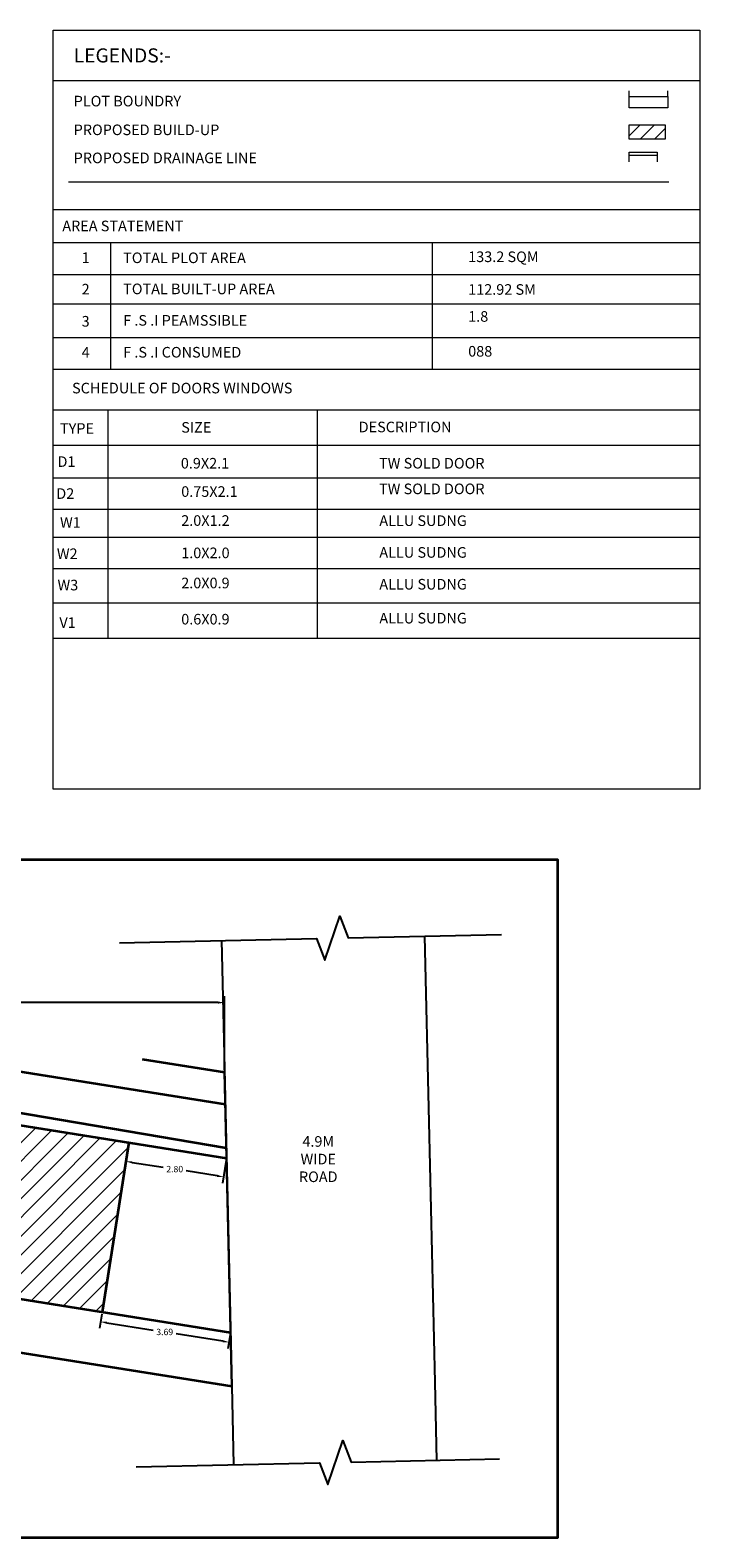
# Model space of a CAD drawing. Units: metres. Extents: x 8.1 to 56.2, y -9.3 to 36.3.
# Tile 6 of 6: x 37.2 to 56.2, y -9.3 to 33.4. Entities that reach past the tile are written whole.
import ezdxf

# ---------------------------------------------------------------- set-up
doc = ezdxf.new("R2010")
doc.units = ezdxf.units.M
doc.header["$LTSCALE"] = 0.01
doc.header["$MEASUREMENT"] = 0
for name, color, linetype, lineweight in [('A-ANNO-DIMS', 2, 'Continuous', 18), ('A-ANNO-SCHD', 7, 'Continuous', 18), ('A-ANNO-TEXT', 7, 'Continuous', 18), ('A-ANNO-TTLB', 7, 'Continuous', 35), ('A-AREA-PATT', 1, 'Continuous', 13), ('C-BLDG', 1, 'Continuous', 35), ('C-PROP', 5, 'Continuous', 35), ('C-ROAD', 8, 'Continuous', 25)]:
    doc.layers.add(name, color=color, linetype=linetype, lineweight=lineweight)
doc.styles.get("Standard").update_dxf_attribs({"font": 'arial.ttf'})
doc.dimstyles.get("Standard").update_dxf_attribs({"dimtxt": 0.18, "dimasz": 0.18, "dimexe": 0.18, "dimexo": 0.0625, "dimgap": 0.09, "dimtad": 0, "dimtih": 1, "dimtoh": 1, "dimzin": 0, "dimdsep": 46, "dimtxsty": 'Standard', "dimcen": 0.09, "dimadec": 0, "dimazin": 0, "dimtfac": 1, "dimtofl": 0, "dimtmove": 0, "dimatfit": 3, "dimfxl": 1, "dimtolj": 1, "dimtzin": 0, "dimarcsym": 0})

# ---------------------------------------------------------------- blocks, each defined once
blk = doc.blocks.new('*D11')
at = {"layer": 'A-ANNO-DIMS', "color": 0, "lineweight": -2, "transparency": 16777216}
for p, q in [((26.382, 5.014), (26.382, 6.024)), ((42.755, 3.933), (42.755, 6.024)), ((26.562, 5.844), (34.183, 5.844)), ((42.575, 5.844), (34.954, 5.844))]:
    blk.add_line(p, q, dxfattribs=at)
at = {"layer": 'A-ANNO-DIMS', "color": 0, "transparency": 16777216}
for points in [[(26.562, 5.874), (26.562, 5.814), (26.382, 5.844)], [(42.575, 5.874), (42.575, 5.814), (42.755, 5.844)]]:
    blk.add_solid(points, dxfattribs=at)
at = {"layer": 'Defpoints', "color": 0, "transparency": 16777216}
for p in [(42.755, 5.844), (26.382, 4.951), (42.755, 3.87)]:
    blk.add_point(p, dxfattribs=at)
at = {"layer": 'A-ANNO-DIMS', "color": 0, "transparency": 16777216, "insert": (34.568, 5.844), "char_height": 0.18, "attachment_point": 5}
blk.add_mtext('\\A1;16.37', dxfattribs=at)
blk = doc.blocks.new('*D15')
at = {"layer": 'A-ANNO-DIMS', "color": 0, "lineweight": -2, "transparency": 16777216}
for p, q in [((39.277, -2.982), (39.215, -3.374)), ((39.421, -3.224), (40.739, -3.434)), ((42.706, -3.746), (41.387, -3.537)), ((42.917, -3.56), (42.855, -3.952))]:
    blk.add_line(p, q, dxfattribs=at)
at = {"layer": 'A-ANNO-DIMS', "color": 0, "transparency": 16777216}
for points in [[(39.426, -3.195), (39.416, -3.254), (39.243, -3.196)], [(42.71, -3.716), (42.701, -3.776), (42.883, -3.774)]]:
    blk.add_solid(points, dxfattribs=at)
at = {"layer": 'Defpoints', "color": 0, "transparency": 16777216}
for p in [(39.287, -2.92), (42.883, -3.774), (42.927, -3.498)]:
    blk.add_point(p, dxfattribs=at)
at = {"layer": 'A-ANNO-DIMS', "color": 0, "transparency": 16777216, "insert": (41.063, -3.485), "char_height": 0.18, "attachment_point": 5}
blk.add_mtext('\\A1;3.69', dxfattribs=at)
blk = doc.blocks.new('*D16')
at = {"layer": 'A-ANNO-DIMS', "color": 0, "lineweight": -2, "transparency": 16777216}
for p, q in [((40.04, 1.818), (39.937, 1.17)), ((40.143, 1.319), (41.021, 1.18)), ((42.802, 1.379), (42.699, 0.731)), ((42.549, 0.937), (41.671, 1.076))]:
    blk.add_line(p, q, dxfattribs=at)
at = {"layer": 'A-ANNO-DIMS', "color": 0, "transparency": 16777216}
for points in [[(40.147, 1.349), (40.138, 1.289), (39.965, 1.347)], [(42.554, 0.967), (42.545, 0.907), (42.727, 0.909)]]:
    blk.add_solid(points, dxfattribs=at)
at = {"layer": 'Defpoints', "color": 0, "transparency": 16777216}
for p in [(40.049, 1.88), (42.812, 1.441), (42.727, 0.909)]:
    blk.add_point(p, dxfattribs=at)
at = {"layer": 'A-ANNO-DIMS', "color": 0, "transparency": 16777216, "insert": (41.346, 1.128), "char_height": 0.18, "attachment_point": 5}
blk.add_mtext('\\A1;2.80', dxfattribs=at)

msp = doc.modelspace()

# ---------------------------------------------------------------- hatches: boundary and pattern name
at = {"layer": 'A-AREA-PATT', "transparency": 33554574}
h = msp.add_hatch(dxfattribs=at)
h.set_pattern_fill('ANSI31', color=256, scale=2.3)
h.set_pattern_definition([(45, (9.19188, 0), (-0.2032932, 0.2032932), [])])
h.paths.add_polyline_path([(55.244, 30.299), (55.244, 30.711), (54.221, 30.711), (54.221, 30.299)])
h = msp.add_hatch(dxfattribs=at)
h.set_pattern_fill('ANSI31', color=256, scale=3)
h.set_pattern_definition([(45, (-0.34318, 4.324), (-0.265165, 0.265165), [])])
h.paths.add_polyline_path([(39.287, -2.92), (40.049, 1.88), (34.41, 2.775), (34.314, 2.173), (27.628, 3.234), (26.962, -0.963)])

# ---------------------------------------------------------------- linework, layer by layer
at = {"layer": 'A-ANNO-SCHD'}
for p, q in [((37.899, 31.964), (56.228, 31.964)), ((54.221, 31.509), (54.221, 31.671)), ((55.324, 31.509), (55.324, 31.671)), ((54.221, 29.933), (55.019, 29.933)), ((54.221, 29.654), (54.221, 29.933)), ((55.019, 29.933), (55.019, 29.654)), ((55.019, 29.84), (54.221, 29.84))]:
    msp.add_line(p, q, dxfattribs=at)
at = {"layer": 'A-ANNO-SCHD', "ltscale": 0.01}
for p, q in [((38.338, 29.088), (55.352, 29.088)), ((37.899, 28.305), (56.228, 28.305)), ((37.899, 27.374), (56.228, 27.374)), ((39.523, 27.374), (39.523, 23.783)), ((48.641, 27.374), (48.641, 23.783)), ((37.899, 26.47), (56.228, 26.47)), ((37.899, 25.636), (56.228, 25.636)), ((37.899, 24.687), (56.228, 24.687)), ((37.899, 23.783), (56.228, 23.783)), ((37.899, 22.638), (56.228, 22.638)), ((39.452, 22.638), (39.452, 16.171)), ((45.387, 22.638), (45.387, 16.171)), ((37.899, 21.629), (56.228, 21.629)), ((37.899, 20.712), (56.228, 20.712)), ((37.899, 19.82), (56.228, 19.82)), ((37.899, 19.027), (56.228, 19.027)), ((37.899, 18.135), (56.228, 18.135)), ((37.899, 17.167), (56.228, 17.167)), ((37.899, 16.171), (56.228, 16.171))]:
    msp.add_line(p, q, dxfattribs=at)
at = {"layer": 'A-ANNO-SCHD'}
for points in [[(37.899, 33.388), (56.228, 33.388), (56.228, 11.889), (37.899, 11.889)], [(54.221, 31.509), (55.324, 31.509), (55.324, 31.184), (54.221, 31.184)], [(54.221, 30.711), (55.244, 30.711), (55.244, 30.299), (54.221, 30.299)]]:
    msp.add_lwpolyline(points, close=True, dxfattribs=at)
at = {"layer": 'A-ANNO-TTLB'}
msp.add_lwpolyline([(22.566, 9.894), (52.195, 9.894), (52.195, -9.317), (22.566, -9.317)], close=True, dxfattribs=at)
at = {"layer": 'C-BLDG'}
msp.add_line((42.805, 1.724), (27.973, 4.24), dxfattribs=at)
at = {"layer": 'C-PROP'}
for p, q in [((34.645, 4.257), (42.776, 2.966)), ((40.424, 4.24), (42.755, 3.87)), ((34.41, 2.775), (42.812, 1.441)), ((40.049, 1.88), (39.287, -2.92)), ((26.962, -0.963), (42.927, -3.498)), ((25.245, -2.209), (42.963, -5.023))]:
    msp.add_line(p, q, dxfattribs=at)
at = {"layer": 'C-ROAD'}
for p, q in [((48.422, 7.722), (48.545, 2.46)), ((42.668, 7.608), (42.791, 2.346)), ((42.963, -5.023), (42.755, 3.87)), ((42.791, 2.346), (42.963, -5.023)), ((48.545, 2.46), (48.718, -4.909)), ((42.963, -5.023), (43.015, -7.237)), ((48.718, -4.909), (48.769, -7.123))]:
    msp.add_line(p, q, dxfattribs=at)
for points in [[(39.785, 7.541), (45.363, 7.66), (45.601, 7.047), (46.025, 8.293), (46.263, 7.679), (50.602, 7.772)], [(40.253, -7.301), (45.449, -7.19), (45.687, -7.803), (46.111, -6.558), (46.349, -7.171), (50.554, -7.081)]]:
    msp.add_lwpolyline(points, dxfattribs=at)

# ---------------------------------------------------------------- texts
at = {"layer": 'A-ANNO-TEXT', "attachment_point": 1}
for s, width, insert, char_height in [('LEGENDS:-', 5.13719, (38.483, 32.872), 0.4), ('PLOT BOUNDRY', 5.13719, (38.483, 31.529), 0.3), ('PROPOSED BUILD-UP', 6.01887, (38.483, 30.715), 0.3), ('PROPOSED DRAINAGE LINE', 8.34819, (38.483, 29.919), 0.3), ('AREA STATEMENT', 8.34819, (38.161, 27.992), 0.3), ('1', 0.4385, (38.709, 27.094), 0.3), ('TOTAL PLOT AREA', 8.34819, (39.885, 27.09), 0.3), ('133.2 SQM', 8.34819, (49.663, 27.119), 0.3), ('2', 0.4385, (38.709, 26.202), 0.3), ('TOTAL BUILT-UP AREA', 8.34819, (39.885, 26.209), 0.3), ('112.92 SM', 8.34819, (49.663, 26.193), 0.3), ('3', 0.4385, (38.709, 25.292), 0.3), ('F .S .I PEAMSSIBLE', 8.34819, (39.885, 25.318), 0.3), ('1.8', 8.34819, (49.663, 25.429), 0.3), ('4', 0.4385, (38.709, 24.412), 0.3), ('F .S .I CONSUMED', 8.34819, (39.885, 24.415), 0.3), ('088', 8.34819, (49.663, 24.442), 0.3), ('SCHEDULE OF DOORS WINDOWS', 8.34819, (38.437, 23.4), 0.3), ('TYPE', 1.34814, (38.096, 22.256), 0.3), ('SIZE', 1.34814, (41.531, 22.288), 0.3), ('DESCRIPTION', 3.42316, (46.56, 22.298), 0.3), ('D1', 1.34814, (38.025, 21.317), 0.3), ('\\pxqc;0.9X2.1', 1.34814, (41.531, 21.271), 0.3), ('TW SOLD DOOR', 5.35119, (47.137, 21.271), 0.3), ('TW SOLD DOOR', 3.28389, (47.137, 20.545), 0.3), ('D2', 1.34814, (37.99, 20.412), 0.3), ('\\pxt4;0.75X2.1', 1.9137, (41.531, 20.469), 0.3), ('2.0X1.2', 1.34814, (41.531, 19.648), 0.3), ('ALLU SUDNG', 2.96439, (47.145, 19.644), 0.3), ('W1', 1.34814, (38.096, 19.593), 0.3), ('W2', 1.34814, (38.007, 18.707), 0.3), ('1.0X2.0', 1.34814, (41.531, 18.732), 0.3), ('ALLU SUDNG', 2.96439, (47.145, 18.745), 0.3), ('W3', 1.34814, (38.025, 17.82), 0.3), ('2.0X0.9', 1.34814, (41.531, 17.879), 0.3), ('ALLU SUDNG', 2.96439, (47.145, 17.844), 0.3), ('V1', 1.34814, (38.078, 16.757), 0.3), ('0.6X0.9', 1.34814, (41.531, 16.854), 0.3), ('ALLU SUDNG', 2.96439, (47.145, 16.883), 0.3), ('\\pxqc;4.9M\\PWIDE\\PROAD', 4.05553, (43.386, 2.061), 0.3)]:
    msp.add_mtext_dynamic_manual_height_columns(s, width=width, gutter_width=1, heights=[0], dxfattribs=dict(at, insert=insert, char_height=char_height))

# ---------------------------------------------------------------- dimensions: what is measured, and where the dimension line sits
at = {"layer": 'A-ANNO-DIMS'}
dim = msp.add_linear_dim(base=(42.755, 5.844), p1=(26.382, 4.951), p2=(42.755, 3.87), dimstyle='Standard', override={"dimclrd": 0, "dimclre": 0, "dimclrt": 0}, dxfattribs=at)
dim.commit()
dim.dimension.update_dxf_attribs({"geometry": '*D11', "text_midpoint": (34.568, 5.844)})
for p1, p2, distance, picture, middle in [((40.049, 1.88), (42.812, 1.441), -0.539, '*D16', (41.346, 1.128)), ((39.287, -2.92), (42.927, -3.498), -0.28, '*D15', (41.063, -3.485))]:
    dim = msp.add_aligned_dim(p1=p1, p2=p2, distance=distance, dimstyle='Standard', override={"dimclrd": 0, "dimclre": 0, "dimclrt": 0}, dxfattribs=at)
    dim.commit()
    dim.dimension.update_dxf_attribs({"geometry": picture, "text_midpoint": middle})

doc.saveas('drawing.dxf')
